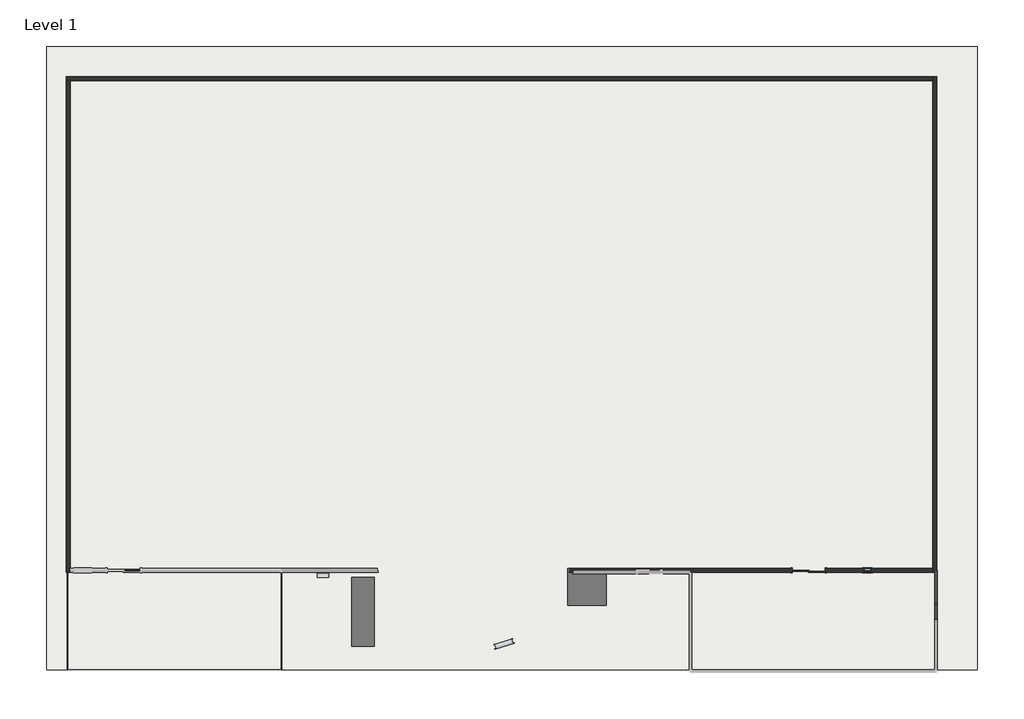
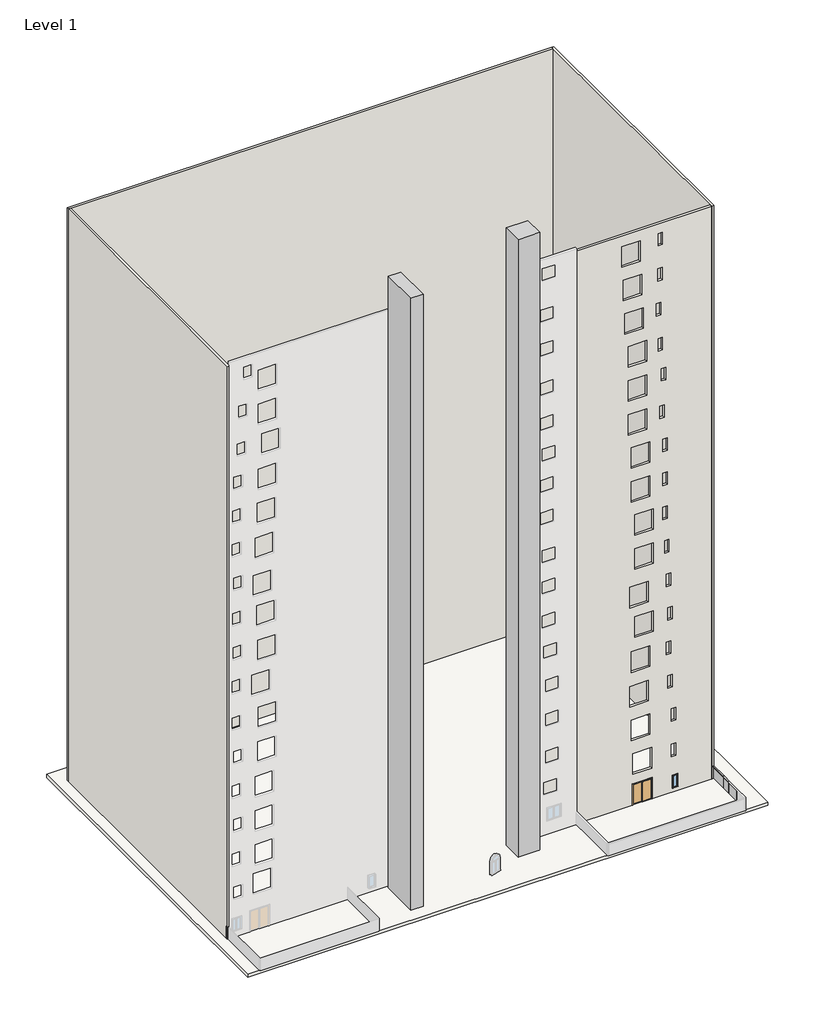
# One storey, part 3 of 3: 4 walls, 3 plates, 2 members, 2 proxies, 1 door, 1 slab, 1 window.
"""IFC4 building model written with IfcOpenShell, lengths in millimetres."""

from ifc_helpers import new_model, si_unit, frame, origin, place, context, project, spatial, polyline, circle_curve, outline, extrude, faceted_brep, transform, mapped, element, save
from ifc_brep_helpers import plane_surface, revolved_surface, advanced_brep
from components import generic_models_1_generic_models_1_ad90d225, generic_models_2_generic_models_2_24f987b9, door_076b30e0, member_ac3a6214, member_afcd4490, system_panel_glazed_8dce6023, system_panel_glazed_2adfbad0, system_panel_glazed_e6c99a0d, window_a765b88f

model = new_model("IFC4")

# Units and contexts
model_context = context("Model", 3, world=origin())
ifc_project = project(units=[si_unit("LENGTHUNIT", "METRE", prefix="MILLI")], contexts=[model_context])

# Site, building, storey
site = spatial("IfcSite", under=ifc_project)
building = spatial("IfcBuilding", under=site)
storey = spatial("IfcBuildingStorey", under=building, Name="Level 1", Elevation=0.0)

# Proxies
placement = place(None, origin())
generic_models_1_generic_models_1_shape = generic_models_1_generic_models_1_ad90d225(model_context)
element("IfcBuildingElementProxy", 1, Name="Generic Models 1 : Generic Models 1", ObjectType="Generic Models 1 : Generic Models 1", at=placement, inside=storey, context=model_context, shape_type="MappedRepresentation", body=[
    mapped(generic_models_1_generic_models_1_shape, transform((0.0, 0.0, 0.0), x_axis=(1.0, 0.0, 0.0), y_axis=(0.0, 1.0, 0.0), z_axis=(0.0, 0.0, 1.0))),
])
generic_models_2_generic_models_2_shape = generic_models_2_generic_models_2_24f987b9(model_context)
element("IfcBuildingElementProxy", 2, Name="Generic Models 2 : Generic Models 2", ObjectType="Generic Models 2 : Generic Models 2", at=placement, inside=storey, context=model_context, shape_type="MappedRepresentation", body=[
    mapped(generic_models_2_generic_models_2_shape, transform((0.0, 0.0, 0.0), x_axis=(1.0, 0.0, 0.0), y_axis=(0.0, 1.0, 0.0), z_axis=(0.0, 0.0, 1.0))),
])

# Door
door_shape = door_076b30e0(model_context)
element("IfcDoor", 3, ObjectType="Door-Double-Sliding : 68\" x 80\"", at=placement, inside=storey, context=model_context, shape_type="MappedRepresentation", body=[
    mapped(door_shape, transform((18835.014721, -12227.7237084, 0.0), x_axis=(-1.0, 0.0, 0.0), y_axis=(0.0, -1.0, 0.0), z_axis=(0.0, 0.0, 1.0))),
])

# Members
member_shape = member_ac3a6214(model_context)
element("IfcMember", 4, ObjectType="Rectangular Mullion : 2.5\" x 5\" rectangular", at=placement, inside=storey, context=model_context, shape_type="MappedRepresentation", body=[
    mapped(member_shape, transform((25464.414721, -14075.656218, 1219.2), x_axis=(0.0, 0.0, 1.0), y_axis=(-1.0, 0.0, 0.0), z_axis=(0.0, -1.0, 0.0))),
])
member_2_shape = member_afcd4490(model_context)
element("IfcMember", 5, ObjectType="Rectangular Mullion : 2.5\" x 5\" rectangular", at=placement, inside=storey, context=model_context, shape_type="MappedRepresentation", body=[
    mapped(member_2_shape, transform((25464.414721, -14936.1224728, 1219.2), x_axis=(0.0, 0.0, 1.0), y_axis=(-1.0, 0.0, 0.0), z_axis=(0.0, -1.0, 0.0))),
])

# Plates
system_panel_glazed_shape = system_panel_glazed_8dce6023(model_context)
element("IfcPlate", 6, ObjectType="System Panel : Glazed", at=placement, inside=storey, context=model_context, shape_type="MappedRepresentation", body=[
    mapped(system_panel_glazed_shape, transform((25464.414721, -13215.1899632, 0.0), x_axis=(0.0, -1.0, 0.0), y_axis=(1.0, 0.0, 0.0), z_axis=(0.0, 0.0, 1.0))),
])
system_panel_glazed_2_shape = system_panel_glazed_2adfbad0(model_context)
element("IfcPlate", 7, ObjectType="System Panel : Glazed", at=placement, inside=storey, context=model_context, shape_type="MappedRepresentation", body=[
    mapped(system_panel_glazed_2_shape, transform((25464.414721, -15581.4721639, 0.0), x_axis=(0.0, -1.0, 0.0), y_axis=(1.0, 0.0, 0.0), z_axis=(0.0, 0.0, 1.0))),
])
system_panel_glazed_3_shape = system_panel_glazed_e6c99a0d(model_context)
element("IfcPlate", 8, ObjectType="System Panel : Glazed", at=placement, inside=storey, context=model_context, shape_type="MappedRepresentation", body=[
    mapped(system_panel_glazed_3_shape, transform((25464.414721, -14505.8893454, 0.0), x_axis=(0.0, -1.0, 0.0), y_axis=(1.0, 0.0, 0.0), z_axis=(0.0, 0.0, 1.0))),
])

# Slab
element("IfcSlab", 9, ObjectType="Generic - 12\"", at=placement, inside=storey, context=model_context, shape_type="SweptSolid", body=[
    extrude(outline(polyline([(27613.7744519, 14926.278145), (27613.7744519, -17534.921855), (-20849.4255481, -17534.921855), (-20849.4255481, 14926.278145), (27613.7744519, 14926.278145)])), frame((0.0, 0.0, -304.8), z_axis=(0.0, 0.0, 1.0), x_axis=(1.0, 0.0, 0.0)), (0.0, 0.0, 1.0), 304.8),
])

# Walls
element("IfcWall", 10, ObjectType="Generic - 8\"", at=placement, inside=storey, context=model_context, shape_type="Brep", body=[
    faceted_brep([(-19823.785279, 13146.8762916, 0.0), (-19620.585279, 13146.8762916, 0.0), (25286.614721, 13146.8762916, 0.0), (25286.614721, 13146.8762916, 56425.3367162), (-19620.585279, 13146.8762916, 56425.3367162), (-19823.785279, 13146.8762916, 56425.3367162), (-19823.785279, 13350.0762916, 0.0), (-19823.785279, 13350.0762916, 56425.3367162), (25286.614721, 13350.0762916, 56425.3367162), (25286.614721, 13350.0762916, 0.0)], [[[0, 1, 2, 3, 4, 5]], [[6, 7, 8, 9]], [[2, 1, 0, 6, 9]], [[5, 4, 3, 8, 7]], [[0, 5, 7, 6]], [[3, 2, 9, 8]]]),
])
element("IfcWall", 11, ObjectType="Generic - 8\"", at=placement, inside=storey, context=model_context, shape_type="Brep", body=[
    faceted_brep([(-19620.585279, -12456.3237084, 0.0), (-19620.585279, -12253.1237084, 0.0), (-19620.585279, 13146.8762916, 0.0), (-19620.585279, 13146.8762916, 56425.3367162), (-19620.585279, -12456.3237084, 56425.3367162), (-19823.785279, -12456.3237084, 0.0), (-19823.785279, -12456.3237084, 56425.3367162), (-19823.785279, 13146.8762916, 56425.3367162), (-19823.785279, 13146.8762916, 0.0)], [[[0, 1, 2, 3, 4]], [[5, 6, 7, 8]], [[2, 1, 0, 5, 8]], [[4, 3, 7, 6]], [[0, 4, 6, 5]], [[3, 2, 8, 7]]]),
])
element("IfcWall", 12, ObjectType="Generic - 8\"", at=placement, inside=storey, context=model_context, shape_type="Brep", body=[
    faceted_brep([(25286.614721, 13350.0762916, 0.0), (25286.614721, 13146.8762916, 0.0), (25286.614721, -12253.1237084, 0.0), (25286.614721, -12456.3237084, 0.0), (25286.614721, -12456.3237084, 56425.3367162), (25286.614721, -12253.1237084, 56425.3367162), (25286.614721, 13146.8762916, 56425.3367162), (25286.614721, 13350.0762916, 56425.3367162), (25489.814721, 13350.0762916, 0.0), (25489.814721, 13350.0762916, 56425.3367162), (25489.814721, -12456.3237084, 56425.3367162), (25489.814721, -12456.3237084, 0.0)], [[[0, 1, 2, 3, 4, 5, 6, 7]], [[8, 9, 10, 11]], [[3, 2, 1, 0, 8, 11]], [[7, 6, 5, 4, 10, 9]], [[0, 7, 9, 8]], [[4, 3, 11, 10]]]),
])
element("IfcWall", 13, ObjectType="Generic - 8\"", at=placement, inside=storey, context=model_context, shape_type="AdvancedBrep", body=[
    advanced_brep(
    [(17971.414721, -12253.1237084, 2032.0), (17971.414721, -12253.1237084, 0.0), (6408.3657946, -12253.1237084, 0.0), (6408.3657946, -12253.1237084, 56425.3367162), (25286.614721, -12253.1237084, 56425.3367162), (25286.614721, -12253.1237084, 0.0), (19698.614721, -12253.1237084, 0.0), (19698.614721, -12253.1237084, 2032.0), (18631.814721, -12253.1237084, 55372.0), (16904.614721, -12253.1237084, 55372.0), (16904.614721, -12253.1237084, 53340.0), (18631.814721, -12253.1237084, 53340.0), (18784.214721, -12253.1237084, 52019.2), (17057.014721, -12253.1237084, 52019.2), (17057.014721, -12253.1237084, 49987.2), (18784.214721, -12253.1237084, 49987.2), (18936.614721, -12253.1237084, 48666.4), (17209.414721, -12253.1237084, 48666.4), (17209.414721, -12253.1237084, 46634.4), (18936.614721, -12253.1237084, 46634.4), (19241.414721, -12253.1237084, 45313.6), (17514.214721, -12253.1237084, 45313.6), (17514.214721, -12253.1237084, 43281.6), (19241.414721, -12253.1237084, 43281.6), (19241.414721, -12253.1237084, 41960.8), (17514.214721, -12253.1237084, 41960.8), (17514.214721, -12253.1237084, 39928.8), (19241.414721, -12253.1237084, 39928.8), (19241.414721, -12253.1237084, 38608.0), (17514.214721, -12253.1237084, 38608.0), (17514.214721, -12253.1237084, 36576.0), (19241.414721, -12253.1237084, 36576.0), (19546.214721, -12253.1237084, 35255.2), (17819.014721, -12253.1237084, 35255.2), (17819.014721, -12253.1237084, 33223.2), (19546.214721, -12253.1237084, 33223.2), (19546.214721, -12253.1237084, 31902.4), (17819.014721, -12253.1237084, 31902.4), (17819.014721, -12253.1237084, 29870.4), (19546.214721, -12253.1237084, 29870.4), (19851.014721, -12253.1237084, 25196.8), (18123.814721, -12253.1237084, 25196.8), (18123.814721, -12253.1237084, 23164.8), (19851.014721, -12253.1237084, 23164.8), (19393.814721, -12253.1237084, 21539.2), (17666.614721, -12253.1237084, 21539.2), (17666.614721, -12253.1237084, 19507.2), (19393.814721, -12253.1237084, 19507.2), (19851.014721, -12253.1237084, 28549.6), (18123.814721, -12253.1237084, 28549.6), (18123.814721, -12253.1237084, 26517.6), (19851.014721, -12253.1237084, 26517.6), (19851.014721, -12253.1237084, 18491.2), (18123.814721, -12253.1237084, 18491.2), (18123.814721, -12253.1237084, 16459.2), (19851.014721, -12253.1237084, 16459.2), (19546.214721, -12253.1237084, 15138.4), (17819.014721, -12253.1237084, 15138.4), (17819.014721, -12253.1237084, 13106.4), (19546.214721, -12253.1237084, 13106.4), (19393.814721, -12253.1237084, 11785.6), (17666.614721, -12253.1237084, 11785.6), (17666.614721, -12253.1237084, 9753.6), (19393.814721, -12253.1237084, 9753.6), (19546.214721, -12253.1237084, 8432.8), (17819.014721, -12253.1237084, 8432.8), (17819.014721, -12253.1237084, 6400.8), (19546.214721, -12253.1237084, 6400.8), (19698.614721, -12253.1237084, 5080.0), (17971.414721, -12253.1237084, 5080.0), (17971.414721, -12253.1237084, 3048.0), (19698.614721, -12253.1237084, 3048.0), (20308.214721, -12253.1237084, 55473.6), (20308.214721, -12253.1237084, 54254.4), (20714.614721, -12253.1237084, 54254.4), (20714.614721, -12253.1237084, 55473.6), (20282.814721, -12253.1237084, 52022.3677442), (20282.814721, -12253.1237084, 50803.1677442), (20689.214721, -12253.1237084, 50803.1677442), (20689.214721, -12253.1237084, 52022.3677442), (20155.814721, -12253.1237084, 48604.1519596), (20155.814721, -12253.1237084, 47384.9519596), (20562.214721, -12253.1237084, 47384.9519596), (20562.214721, -12253.1237084, 48604.1519596), (20308.214721, -12253.1237084, 45110.4), (20308.214721, -12253.1237084, 43891.2), (20714.614721, -12253.1237084, 43891.2), (20714.614721, -12253.1237084, 45110.4), (20613.014721, -12253.1237084, 42062.4), (20613.014721, -12253.1237084, 40843.2), (21019.414721, -12253.1237084, 40843.2), (21019.414721, -12253.1237084, 42062.4), (20460.614721, -12253.1237084, 38404.8), (20460.614721, -12253.1237084, 37185.6), (20867.014721, -12253.1237084, 37185.6), (20867.014721, -12253.1237084, 38404.8), (20765.414721, -12253.1237084, 35052.0), (20765.414721, -12253.1237084, 33832.8), (21171.814721, -12253.1237084, 33832.8), (21171.814721, -12253.1237084, 35052.0), (20765.414721, -12253.1237084, 31699.2), (20765.414721, -12253.1237084, 30480.0), (21171.814721, -12253.1237084, 30480.0), (21171.814721, -12253.1237084, 31699.2), (20765.414721, -12253.1237084, 28346.4), (20765.414721, -12253.1237084, 27127.2), (21171.814721, -12253.1237084, 27127.2), (21171.814721, -12253.1237084, 28346.4), (20917.814721, -12253.1237084, 24993.6), (20917.814721, -12253.1237084, 23774.4), (21324.214721, -12253.1237084, 23774.4), (21324.214721, -12253.1237084, 24993.6), (21070.214721, -12253.1237084, 21640.8), (21070.214721, -12253.1237084, 20421.6), (21476.614721, -12253.1237084, 20421.6), (21476.614721, -12253.1237084, 21640.8), (21222.614721, -12253.1237084, 18288.0), (21222.614721, -12253.1237084, 17068.8), (21629.014721, -12253.1237084, 17068.8), (21629.014721, -12253.1237084, 18288.0), (21070.214721, -12253.1237084, 14935.2), (21070.214721, -12253.1237084, 13716.0), (21476.614721, -12253.1237084, 13716.0), (21476.614721, -12253.1237084, 14935.2), (21222.614721, -12253.1237084, 11582.4), (21222.614721, -12253.1237084, 10363.2), (21629.014721, -12253.1237084, 10363.2), (21629.014721, -12253.1237084, 11582.4), (21527.414721, -12253.1237084, 8229.6), (21527.414721, -12253.1237084, 7010.4), (21933.814721, -12253.1237084, 7010.4), (21933.814721, -12253.1237084, 8229.6), (21527.414721, -12253.1237084, 4734.0057153), (21527.414721, -12253.1237084, 3514.8057153), (21933.814721, -12253.1237084, 3514.8057153), (21933.814721, -12253.1237084, 4734.0057153), (21679.814721, -12253.1237084, 1610.6543351), (21679.814721, -12253.1237084, 391.4543351), (22086.214721, -12253.1237084, 391.4543351), (22086.214721, -12253.1237084, 1610.6543351), (6362.4838197, -12456.3237084, 0.0), (6571.5594464, -12456.3237084, 0.0), (17971.414721, -12456.3237084, 0.0), (17971.414721, -12456.3237084, 2032.0), (19698.614721, -12456.3237084, 2032.0), (19698.614721, -12456.3237084, 0.0), (25286.614721, -12456.3237084, 0.0), (25286.614721, -12456.3237084, 56425.3367162), (6571.5594464, -12456.3237084, 56425.3367162), (6362.4838197, -12456.3237084, 56425.3367162), (18631.814721, -12456.3237084, 55372.0), (18631.814721, -12456.3237084, 53340.0), (16904.614721, -12456.3237084, 53340.0), (16904.614721, -12456.3237084, 55372.0), (18784.214721, -12456.3237084, 52019.2), (18784.214721, -12456.3237084, 49987.2), (17057.014721, -12456.3237084, 49987.2), (17057.014721, -12456.3237084, 52019.2), (18936.614721, -12456.3237084, 48666.4), (18936.614721, -12456.3237084, 46634.4), (17209.414721, -12456.3237084, 46634.4), (17209.414721, -12456.3237084, 48666.4), (19241.414721, -12456.3237084, 45313.6), (19241.414721, -12456.3237084, 43281.6), (17514.214721, -12456.3237084, 43281.6), (17514.214721, -12456.3237084, 45313.6), (19241.414721, -12456.3237084, 41960.8), (19241.414721, -12456.3237084, 39928.8), (17514.214721, -12456.3237084, 39928.8), (17514.214721, -12456.3237084, 41960.8), (19241.414721, -12456.3237084, 38608.0), (19241.414721, -12456.3237084, 36576.0), (17514.214721, -12456.3237084, 36576.0), (17514.214721, -12456.3237084, 38608.0), (19546.214721, -12456.3237084, 35255.2), (19546.214721, -12456.3237084, 33223.2), (17819.014721, -12456.3237084, 33223.2), (17819.014721, -12456.3237084, 35255.2), (19546.214721, -12456.3237084, 31902.4), (19546.214721, -12456.3237084, 29870.4), (17819.014721, -12456.3237084, 29870.4), (17819.014721, -12456.3237084, 31902.4), (19851.014721, -12456.3237084, 25196.8), (19851.014721, -12456.3237084, 23164.8), (18123.814721, -12456.3237084, 23164.8), (18123.814721, -12456.3237084, 25196.8), (19393.814721, -12456.3237084, 21539.2), (19393.814721, -12456.3237084, 19507.2), (17666.614721, -12456.3237084, 19507.2), (17666.614721, -12456.3237084, 21539.2), (19851.014721, -12456.3237084, 28549.6), (19851.014721, -12456.3237084, 26517.6), (18123.814721, -12456.3237084, 26517.6), (18123.814721, -12456.3237084, 28549.6), (19851.014721, -12456.3237084, 18491.2), (19851.014721, -12456.3237084, 16459.2), (18123.814721, -12456.3237084, 16459.2), (18123.814721, -12456.3237084, 18491.2), (19546.214721, -12456.3237084, 15138.4), (19546.214721, -12456.3237084, 13106.4), (17819.014721, -12456.3237084, 13106.4), (17819.014721, -12456.3237084, 15138.4), (19393.814721, -12456.3237084, 11785.6), (19393.814721, -12456.3237084, 9753.6), (17666.614721, -12456.3237084, 9753.6), (17666.614721, -12456.3237084, 11785.6), (19546.214721, -12456.3237084, 8432.8), (19546.214721, -12456.3237084, 6400.8), (17819.014721, -12456.3237084, 6400.8), (17819.014721, -12456.3237084, 8432.8), (19698.614721, -12456.3237084, 5080.0), (19698.614721, -12456.3237084, 3048.0), (17971.414721, -12456.3237084, 3048.0), (17971.414721, -12456.3237084, 5080.0), (20308.214721, -12456.3237084, 55473.6), (20714.614721, -12456.3237084, 55473.6), (20714.614721, -12456.3237084, 54254.4), (20308.214721, -12456.3237084, 54254.4), (20282.814721, -12456.3237084, 52022.3677442), (20689.214721, -12456.3237084, 52022.3677442), (20689.214721, -12456.3237084, 50803.1677442), (20282.814721, -12456.3237084, 50803.1677442), (20155.814721, -12456.3237084, 48604.1519596), (20562.214721, -12456.3237084, 48604.1519596), (20562.214721, -12456.3237084, 47384.9519596), (20155.814721, -12456.3237084, 47384.9519596), (20308.214721, -12456.3237084, 45110.4), (20714.614721, -12456.3237084, 45110.4), (20714.614721, -12456.3237084, 43891.2), (20308.214721, -12456.3237084, 43891.2), (20613.014721, -12456.3237084, 42062.4), (21019.414721, -12456.3237084, 42062.4), (21019.414721, -12456.3237084, 40843.2), (20613.014721, -12456.3237084, 40843.2), (20460.614721, -12456.3237084, 38404.8), (20867.014721, -12456.3237084, 38404.8), (20867.014721, -12456.3237084, 37185.6), (20460.614721, -12456.3237084, 37185.6), (20765.414721, -12456.3237084, 35052.0), (21171.814721, -12456.3237084, 35052.0), (21171.814721, -12456.3237084, 33832.8), (20765.414721, -12456.3237084, 33832.8), (20765.414721, -12456.3237084, 31699.2), (21171.814721, -12456.3237084, 31699.2), (21171.814721, -12456.3237084, 30480.0), (20765.414721, -12456.3237084, 30480.0), (20765.414721, -12456.3237084, 28346.4), (21171.814721, -12456.3237084, 28346.4), (21171.814721, -12456.3237084, 27127.2), (20765.414721, -12456.3237084, 27127.2), (20917.814721, -12456.3237084, 24993.6), (21324.214721, -12456.3237084, 24993.6), (21324.214721, -12456.3237084, 23774.4), (20917.814721, -12456.3237084, 23774.4), (21070.214721, -12456.3237084, 21640.8), (21476.614721, -12456.3237084, 21640.8), (21476.614721, -12456.3237084, 20421.6), (21070.214721, -12456.3237084, 20421.6), (21222.614721, -12456.3237084, 18288.0), (21629.014721, -12456.3237084, 18288.0), (21629.014721, -12456.3237084, 17068.8), (21222.614721, -12456.3237084, 17068.8), (21070.214721, -12456.3237084, 14935.2), (21476.614721, -12456.3237084, 14935.2), (21476.614721, -12456.3237084, 13716.0), (21070.214721, -12456.3237084, 13716.0), (21222.614721, -12456.3237084, 11582.4), (21629.014721, -12456.3237084, 11582.4), (21629.014721, -12456.3237084, 10363.2), (21222.614721, -12456.3237084, 10363.2), (21527.414721, -12456.3237084, 8229.6), (21933.814721, -12456.3237084, 8229.6), (21933.814721, -12456.3237084, 7010.4), (21527.414721, -12456.3237084, 7010.4), (21527.414721, -12456.3237084, 4734.0057153), (21933.814721, -12456.3237084, 4734.0057153), (21933.814721, -12456.3237084, 3514.8057153), (21527.414721, -12456.3237084, 3514.8057153), (21679.814721, -12456.3237084, 1610.6543351), (22086.214721, -12456.3237084, 1610.6543351), (22086.214721, -12456.3237084, 391.4543351), (21679.814721, -12456.3237084, 391.4543351), (6386.5095252, -12354.7237244, 56425.3367162)],
    [
        (0, 1),
        (1, 2),
        (2, 3),
        (3, 4),
        (4, 5),
        (5, 6),
        (6, 7),
        (7, 0),
        (8, 9),
        (9, 10),
        (10, 11),
        (11, 8),
        (12, 13),
        (13, 14),
        (14, 15),
        (15, 12),
        (16, 17),
        (17, 18),
        (18, 19),
        (19, 16),
        (20, 21),
        (21, 22),
        (22, 23),
        (23, 20),
        (24, 25),
        (25, 26),
        (26, 27),
        (27, 24),
        (28, 29),
        (29, 30),
        (30, 31),
        (31, 28),
        (32, 33),
        (33, 34),
        (34, 35),
        (35, 32),
        (36, 37),
        (37, 38),
        (38, 39),
        (39, 36),
        (40, 41),
        (41, 42),
        (42, 43),
        (43, 40),
        (44, 45),
        (45, 46),
        (46, 47),
        (47, 44),
        (48, 49),
        (49, 50),
        (50, 51),
        (51, 48),
        (52, 53),
        (53, 54),
        (54, 55),
        (55, 52),
        (56, 57),
        (57, 58),
        (58, 59),
        (59, 56),
        (60, 61),
        (61, 62),
        (62, 63),
        (63, 60),
        (64, 65),
        (65, 66),
        (66, 67),
        (67, 64),
        (68, 69),
        (69, 70),
        (70, 71),
        (71, 68),
        (72, 73),
        (73, 74),
        (74, 75),
        (75, 72),
        (76, 77),
        (77, 78),
        (78, 79),
        (79, 76),
        (80, 81),
        (81, 82),
        (82, 83),
        (83, 80),
        (84, 85),
        (85, 86),
        (86, 87),
        (87, 84),
        (88, 89),
        (89, 90),
        (90, 91),
        (91, 88),
        (92, 93),
        (93, 94),
        (94, 95),
        (95, 92),
        (96, 97),
        (97, 98),
        (98, 99),
        (99, 96),
        (100, 101),
        (101, 102),
        (102, 103),
        (103, 100),
        (104, 105),
        (105, 106),
        (106, 107),
        (107, 104),
        (108, 109),
        (109, 110),
        (110, 111),
        (111, 108),
        (112, 113),
        (113, 114),
        (114, 115),
        (115, 112),
        (116, 117),
        (117, 118),
        (118, 119),
        (119, 116),
        (120, 121),
        (121, 122),
        (122, 123),
        (123, 120),
        (124, 125),
        (125, 126),
        (126, 127),
        (127, 124),
        (128, 129),
        (129, 130),
        (130, 131),
        (131, 128),
        (132, 133),
        (133, 134),
        (134, 135),
        (135, 132),
        (136, 137),
        (137, 138),
        (138, 139),
        (139, 136),
        (140, 141),
        (141, 142),
        (142, 143),
        (143, 144),
        (144, 145),
        (145, 146),
        (146, 147),
        (147, 148),
        (148, 149),
        (149, 140),
        (150, 151),
        (151, 152),
        (152, 153),
        (153, 150),
        (154, 155),
        (155, 156),
        (156, 157),
        (157, 154),
        (158, 159),
        (159, 160),
        (160, 161),
        (161, 158),
        (162, 163),
        (163, 164),
        (164, 165),
        (165, 162),
        (166, 167),
        (167, 168),
        (168, 169),
        (169, 166),
        (170, 171),
        (171, 172),
        (172, 173),
        (173, 170),
        (174, 175),
        (175, 176),
        (176, 177),
        (177, 174),
        (178, 179),
        (179, 180),
        (180, 181),
        (181, 178),
        (182, 183),
        (183, 184),
        (184, 185),
        (185, 182),
        (186, 187),
        (187, 188),
        (188, 189),
        (189, 186),
        (190, 191),
        (191, 192),
        (192, 193),
        (193, 190),
        (194, 195),
        (195, 196),
        (196, 197),
        (197, 194),
        (198, 199),
        (199, 200),
        (200, 201),
        (201, 198),
        (202, 203),
        (203, 204),
        (204, 205),
        (205, 202),
        (206, 207),
        (207, 208),
        (208, 209),
        (209, 206),
        (210, 211),
        (211, 212),
        (212, 213),
        (213, 210),
        (214, 215),
        (215, 216),
        (216, 217),
        (217, 214),
        (218, 219),
        (219, 220),
        (220, 221),
        (221, 218),
        (222, 223),
        (223, 224),
        (224, 225),
        (225, 222),
        (226, 227),
        (227, 228),
        (228, 229),
        (229, 226),
        (230, 231),
        (231, 232),
        (232, 233),
        (233, 230),
        (234, 235),
        (235, 236),
        (236, 237),
        (237, 234),
        (238, 239),
        (239, 240),
        (240, 241),
        (241, 238),
        (242, 243),
        (243, 244),
        (244, 245),
        (245, 242),
        (246, 247),
        (247, 248),
        (248, 249),
        (249, 246),
        (250, 251),
        (251, 252),
        (252, 253),
        (253, 250),
        (254, 255),
        (255, 256),
        (256, 257),
        (257, 254),
        (258, 259),
        (259, 260),
        (260, 261),
        (261, 258),
        (262, 263),
        (263, 264),
        (264, 265),
        (265, 262),
        (266, 267),
        (267, 268),
        (268, 269),
        (269, 266),
        (270, 271),
        (271, 272),
        (272, 273),
        (273, 270),
        (274, 275),
        (275, 276),
        (276, 277),
        (277, 274),
        (278, 279),
        (279, 280),
        (280, 281),
        (281, 278),
        (5, 146),
        (145, 6),
        (1, 142),
        (140, 2, circle_curve(frame((1385.214721, -11225.6906671, 0.0), z_axis=(0.0, 0.0, 1.0), x_axis=(1.0, 0.0, 0.0)), 5127.1498284)),
        (3, 282, circle_curve(frame((1385.214721, -11225.6906671, 56425.3367162), z_axis=(0.0, 0.0, -1.0), x_axis=(1.0, 0.0, 0.0)), 5127.1498284)),
        (282, 149, circle_curve(frame((1385.214721, -11225.6906671, 56425.3367162), z_axis=(0.0, 0.0, -1.0), x_axis=(1.0, 0.0, 0.0)), 5127.1498284)),
        (147, 4),
        (150, 8),
        (11, 151),
        (10, 152),
        (9, 153),
        (154, 12),
        (15, 155),
        (14, 156),
        (13, 157),
        (158, 16),
        (19, 159),
        (18, 160),
        (17, 161),
        (162, 20),
        (23, 163),
        (22, 164),
        (21, 165),
        (166, 24),
        (27, 167),
        (26, 168),
        (25, 169),
        (170, 28),
        (31, 171),
        (30, 172),
        (29, 173),
        (174, 32),
        (35, 175),
        (34, 176),
        (33, 177),
        (178, 36),
        (39, 179),
        (38, 180),
        (37, 181),
        (182, 40),
        (43, 183),
        (42, 184),
        (41, 185),
        (186, 44),
        (47, 187),
        (46, 188),
        (45, 189),
        (190, 48),
        (51, 191),
        (50, 192),
        (49, 193),
        (194, 52),
        (55, 195),
        (54, 196),
        (53, 197),
        (198, 56),
        (59, 199),
        (58, 200),
        (57, 201),
        (202, 60),
        (63, 203),
        (62, 204),
        (61, 205),
        (206, 64),
        (67, 207),
        (66, 208),
        (65, 209),
        (210, 68),
        (71, 211),
        (70, 212),
        (69, 213),
        (144, 7),
        (0, 143),
        (72, 214),
        (217, 73),
        (216, 74),
        (215, 75),
        (76, 218),
        (221, 77),
        (220, 78),
        (219, 79),
        (80, 222),
        (225, 81),
        (224, 82),
        (223, 83),
        (84, 226),
        (229, 85),
        (228, 86),
        (227, 87),
        (88, 230),
        (233, 89),
        (232, 90),
        (231, 91),
        (92, 234),
        (237, 93),
        (236, 94),
        (235, 95),
        (96, 238),
        (241, 97),
        (240, 98),
        (239, 99),
        (100, 242),
        (245, 101),
        (244, 102),
        (243, 103),
        (104, 246),
        (249, 105),
        (248, 106),
        (247, 107),
        (108, 250),
        (253, 109),
        (252, 110),
        (251, 111),
        (112, 254),
        (257, 113),
        (256, 114),
        (255, 115),
        (116, 258),
        (261, 117),
        (260, 118),
        (259, 119),
        (120, 262),
        (265, 121),
        (264, 122),
        (263, 123),
        (124, 266),
        (269, 125),
        (268, 126),
        (267, 127),
        (128, 270),
        (273, 129),
        (272, 130),
        (271, 131),
        (132, 274),
        (277, 133),
        (276, 134),
        (275, 135),
        (136, 278),
        (281, 137),
        (280, 138),
        (279, 139),
    ],
    [
        plane_surface(frame((25388.214721, -12253.1237084, 0.0), z_axis=(0.0, 1.0, 0.0), x_axis=(-1.0, 0.0, 0.0))),
        plane_surface(frame((25388.214721, -12456.3237084, 0.0), z_axis=(0.0, -1.0, 0.0), x_axis=(1.0, 0.0, 0.0))),
        plane_surface(frame((25489.814721, -12253.1237084, 0.0), z_axis=(0.0, 0.0, -1.0), x_axis=(0.0, -1.0, 0.0))),
        plane_surface(frame((6490.614721, -12253.1237084, 56425.3367162), z_axis=(0.0, 0.0, 1.0), x_axis=(0.0, -1.0, 0.0))),
        plane_surface(frame((25286.614721, 13248.4762916, 0.0), z_axis=(1.0, 0.0, 0.0), x_axis=(0.0, -1.0, 0.0))),
        revolved_surface(polyline([(6512.3645494, -11225.6906671, 0.0), (6512.3645494, -11225.6906671, 56425.3367162)]), (1385.214721, -11225.6906671, 0.0), (0.0, 0.0, -1.0)),
        plane_surface(frame((18631.814721, -12456.3237084, 55372.0), z_axis=(-1.0, 0.0, 0.0), x_axis=(0.0, 1.0, 0.0))),
        plane_surface(frame((18631.814721, -12456.3237084, 53340.0), z_axis=(0.0, 0.0, 1.0), x_axis=(0.0, 1.0, 0.0))),
        plane_surface(frame((16904.614721, -12456.3237084, 53340.0), z_axis=(1.0, 0.0, 0.0), x_axis=(0.0, 1.0, 0.0))),
        plane_surface(frame((16904.614721, -12456.3237084, 55372.0), z_axis=(0.0, 0.0, -1.0), x_axis=(0.0, 1.0, 0.0))),
        plane_surface(frame((18784.214721, -12456.3237084, 52019.2), z_axis=(-1.0, 0.0, 0.0), x_axis=(0.0, 1.0, 0.0))),
        plane_surface(frame((18784.214721, -12456.3237084, 49987.2), z_axis=(0.0, 0.0, 1.0), x_axis=(0.0, 1.0, 0.0))),
        plane_surface(frame((17057.014721, -12456.3237084, 49987.2), z_axis=(1.0, 0.0, 0.0), x_axis=(0.0, 1.0, 0.0))),
        plane_surface(frame((17057.014721, -12456.3237084, 52019.2), z_axis=(0.0, 0.0, -1.0), x_axis=(0.0, 1.0, 0.0))),
        plane_surface(frame((18936.614721, -12456.3237084, 48666.4), z_axis=(-1.0, 0.0, 0.0), x_axis=(0.0, 1.0, 0.0))),
        plane_surface(frame((18936.614721, -12456.3237084, 46634.4), z_axis=(0.0, 0.0, 1.0), x_axis=(0.0, 1.0, 0.0))),
        plane_surface(frame((17209.414721, -12456.3237084, 46634.4), z_axis=(1.0, 0.0, 0.0), x_axis=(0.0, 1.0, 0.0))),
        plane_surface(frame((17209.414721, -12456.3237084, 48666.4), z_axis=(0.0, 0.0, -1.0), x_axis=(0.0, 1.0, 0.0))),
        plane_surface(frame((19241.414721, -12456.3237084, 45313.6), z_axis=(-1.0, 0.0, 0.0), x_axis=(0.0, 1.0, 0.0))),
        plane_surface(frame((19241.414721, -12456.3237084, 43281.6), z_axis=(0.0, 0.0, 1.0), x_axis=(0.0, 1.0, 0.0))),
        plane_surface(frame((17514.214721, -12456.3237084, 43281.6), z_axis=(1.0, 0.0, 0.0), x_axis=(0.0, 1.0, 0.0))),
        plane_surface(frame((17514.214721, -12456.3237084, 45313.6), z_axis=(0.0, 0.0, -1.0), x_axis=(0.0, 1.0, 0.0))),
        plane_surface(frame((19241.414721, -12456.3237084, 41960.8), z_axis=(-1.0, 0.0, 0.0), x_axis=(0.0, 1.0, 0.0))),
        plane_surface(frame((19241.414721, -12456.3237084, 39928.8), z_axis=(0.0, 0.0, 1.0), x_axis=(0.0, 1.0, 0.0))),
        plane_surface(frame((17514.214721, -12456.3237084, 39928.8), z_axis=(1.0, 0.0, 0.0), x_axis=(0.0, 1.0, 0.0))),
        plane_surface(frame((17514.214721, -12456.3237084, 41960.8), z_axis=(0.0, 0.0, -1.0), x_axis=(0.0, 1.0, 0.0))),
        plane_surface(frame((19241.414721, -12456.3237084, 38608.0), z_axis=(-1.0, 0.0, 0.0), x_axis=(0.0, 1.0, 0.0))),
        plane_surface(frame((19241.414721, -12456.3237084, 36576.0), z_axis=(0.0, 0.0, 1.0), x_axis=(0.0, 1.0, 0.0))),
        plane_surface(frame((17514.214721, -12456.3237084, 36576.0), z_axis=(1.0, 0.0, 0.0), x_axis=(0.0, 1.0, 0.0))),
        plane_surface(frame((17514.214721, -12456.3237084, 38608.0), z_axis=(0.0, 0.0, -1.0), x_axis=(0.0, 1.0, 0.0))),
        plane_surface(frame((19546.214721, -12456.3237084, 35255.2), z_axis=(-1.0, 0.0, 0.0), x_axis=(0.0, 1.0, 0.0))),
        plane_surface(frame((19546.214721, -12456.3237084, 33223.2), z_axis=(0.0, 0.0, 1.0), x_axis=(0.0, 1.0, 0.0))),
        plane_surface(frame((17819.014721, -12456.3237084, 33223.2), z_axis=(1.0, 0.0, 0.0), x_axis=(0.0, 1.0, 0.0))),
        plane_surface(frame((17819.014721, -12456.3237084, 35255.2), z_axis=(0.0, 0.0, -1.0), x_axis=(0.0, 1.0, 0.0))),
        plane_surface(frame((19546.214721, -12456.3237084, 31902.4), z_axis=(-1.0, 0.0, 0.0), x_axis=(0.0, 1.0, 0.0))),
        plane_surface(frame((19546.214721, -12456.3237084, 29870.4), z_axis=(0.0, 0.0, 1.0), x_axis=(0.0, 1.0, 0.0))),
        plane_surface(frame((17819.014721, -12456.3237084, 29870.4), z_axis=(1.0, 0.0, 0.0), x_axis=(0.0, 1.0, 0.0))),
        plane_surface(frame((17819.014721, -12456.3237084, 31902.4), z_axis=(0.0, 0.0, -1.0), x_axis=(0.0, 1.0, 0.0))),
        plane_surface(frame((19851.014721, -12456.3237084, 25196.8), z_axis=(-1.0, 0.0, 0.0), x_axis=(0.0, 1.0, 0.0))),
        plane_surface(frame((19851.014721, -12456.3237084, 23164.8), z_axis=(0.0, 0.0, 1.0), x_axis=(0.0, 1.0, 0.0))),
        plane_surface(frame((18123.814721, -12456.3237084, 23164.8), z_axis=(1.0, 0.0, 0.0), x_axis=(0.0, 1.0, 0.0))),
        plane_surface(frame((18123.814721, -12456.3237084, 25196.8), z_axis=(0.0, 0.0, -1.0), x_axis=(0.0, 1.0, 0.0))),
        plane_surface(frame((19393.814721, -12456.3237084, 21539.2), z_axis=(-1.0, 0.0, 0.0), x_axis=(0.0, 1.0, 0.0))),
        plane_surface(frame((19393.814721, -12456.3237084, 19507.2), z_axis=(0.0, 0.0, 1.0), x_axis=(0.0, 1.0, 0.0))),
        plane_surface(frame((17666.614721, -12456.3237084, 19507.2), z_axis=(1.0, 0.0, 0.0), x_axis=(0.0, 1.0, 0.0))),
        plane_surface(frame((17666.614721, -12456.3237084, 21539.2), z_axis=(0.0, 0.0, -1.0), x_axis=(0.0, 1.0, 0.0))),
        plane_surface(frame((19851.014721, -12456.3237084, 28549.6), z_axis=(-1.0, 0.0, 0.0), x_axis=(0.0, 1.0, 0.0))),
        plane_surface(frame((19851.014721, -12456.3237084, 26517.6), z_axis=(0.0, 0.0, 1.0), x_axis=(0.0, 1.0, 0.0))),
        plane_surface(frame((18123.814721, -12456.3237084, 26517.6), z_axis=(1.0, 0.0, 0.0), x_axis=(0.0, 1.0, 0.0))),
        plane_surface(frame((18123.814721, -12456.3237084, 28549.6), z_axis=(0.0, 0.0, -1.0), x_axis=(0.0, 1.0, 0.0))),
        plane_surface(frame((19851.014721, -12456.3237084, 18491.2), z_axis=(-1.0, 0.0, 0.0), x_axis=(0.0, 1.0, 0.0))),
        plane_surface(frame((19851.014721, -12456.3237084, 16459.2), z_axis=(0.0, 0.0, 1.0), x_axis=(0.0, 1.0, 0.0))),
        plane_surface(frame((18123.814721, -12456.3237084, 16459.2), z_axis=(1.0, 0.0, 0.0), x_axis=(0.0, 1.0, 0.0))),
        plane_surface(frame((18123.814721, -12456.3237084, 18491.2), z_axis=(0.0, 0.0, -1.0), x_axis=(0.0, 1.0, 0.0))),
        plane_surface(frame((19546.214721, -12456.3237084, 15138.4), z_axis=(-1.0, 0.0, 0.0), x_axis=(0.0, 1.0, 0.0))),
        plane_surface(frame((19546.214721, -12456.3237084, 13106.4), z_axis=(0.0, 0.0, 1.0), x_axis=(0.0, 1.0, 0.0))),
        plane_surface(frame((17819.014721, -12456.3237084, 13106.4), z_axis=(1.0, 0.0, 0.0), x_axis=(0.0, 1.0, 0.0))),
        plane_surface(frame((17819.014721, -12456.3237084, 15138.4), z_axis=(0.0, 0.0, -1.0), x_axis=(0.0, 1.0, 0.0))),
        plane_surface(frame((19393.814721, -12456.3237084, 11785.6), z_axis=(-1.0, 0.0, 0.0), x_axis=(0.0, 1.0, 0.0))),
        plane_surface(frame((19393.814721, -12456.3237084, 9753.6), z_axis=(0.0, 0.0, 1.0), x_axis=(0.0, 1.0, 0.0))),
        plane_surface(frame((17666.614721, -12456.3237084, 9753.6), z_axis=(1.0, 0.0, 0.0), x_axis=(0.0, 1.0, 0.0))),
        plane_surface(frame((17666.614721, -12456.3237084, 11785.6), z_axis=(0.0, 0.0, -1.0), x_axis=(0.0, 1.0, 0.0))),
        plane_surface(frame((19546.214721, -12456.3237084, 8432.8), z_axis=(-1.0, 0.0, 0.0), x_axis=(0.0, 1.0, 0.0))),
        plane_surface(frame((19546.214721, -12456.3237084, 6400.8), z_axis=(0.0, 0.0, 1.0), x_axis=(0.0, 1.0, 0.0))),
        plane_surface(frame((17819.014721, -12456.3237084, 6400.8), z_axis=(1.0, 0.0, 0.0), x_axis=(0.0, 1.0, 0.0))),
        plane_surface(frame((17819.014721, -12456.3237084, 8432.8), z_axis=(0.0, 0.0, -1.0), x_axis=(0.0, 1.0, 0.0))),
        plane_surface(frame((19698.614721, -12456.3237084, 5080.0), z_axis=(-1.0, 0.0, 0.0), x_axis=(0.0, 1.0, 0.0))),
        plane_surface(frame((19698.614721, -12456.3237084, 3048.0), z_axis=(0.0, 0.0, 1.0), x_axis=(0.0, 1.0, 0.0))),
        plane_surface(frame((17971.414721, -12456.3237084, 3048.0), z_axis=(1.0, 0.0, 0.0), x_axis=(0.0, 1.0, 0.0))),
        plane_surface(frame((17971.414721, -12456.3237084, 5080.0), z_axis=(0.0, 0.0, -1.0), x_axis=(0.0, 1.0, 0.0))),
        plane_surface(frame((19698.614721, -12456.3237084, 2032.0), z_axis=(-1.0, 0.0, 0.0), x_axis=(0.0, 1.0, 0.0))),
        plane_surface(frame((17971.414721, -12456.3237084, 0.0), z_axis=(1.0, 0.0, 0.0), x_axis=(0.0, 1.0, 0.0))),
        plane_surface(frame((17971.414721, -12456.3237084, 2032.0), z_axis=(0.0, 0.0, -1.0), x_axis=(0.0, 1.0, 0.0))),
        plane_surface(frame((20308.214721, -12253.1237084, 55473.6), z_axis=(1.0, 0.0, 0.0), x_axis=(0.0, -1.0, 0.0))),
        plane_surface(frame((20308.214721, -12253.1237084, 54254.4), z_axis=(0.0, 0.0, 1.0), x_axis=(0.0, -1.0, 0.0))),
        plane_surface(frame((20714.614721, -12253.1237084, 54254.4), z_axis=(-1.0, 0.0, 0.0), x_axis=(0.0, -1.0, 0.0))),
        plane_surface(frame((20714.614721, -12253.1237084, 55473.6), z_axis=(0.0, 0.0, -1.0), x_axis=(0.0, -1.0, 0.0))),
        plane_surface(frame((20282.814721, -12253.1237084, 52022.3677442), z_axis=(1.0, 0.0, 0.0), x_axis=(0.0, -1.0, 0.0))),
        plane_surface(frame((20282.814721, -12253.1237084, 50803.1677442), z_axis=(0.0, 0.0, 1.0), x_axis=(0.0, -1.0, 0.0))),
        plane_surface(frame((20689.214721, -12253.1237084, 50803.1677442), z_axis=(-1.0, 0.0, 0.0), x_axis=(0.0, -1.0, 0.0))),
        plane_surface(frame((20689.214721, -12253.1237084, 52022.3677442), z_axis=(0.0, 0.0, -1.0), x_axis=(0.0, -1.0, 0.0))),
        plane_surface(frame((20155.814721, -12253.1237084, 48604.1519596), z_axis=(1.0, 0.0, 0.0), x_axis=(0.0, -1.0, 0.0))),
        plane_surface(frame((20155.814721, -12253.1237084, 47384.9519596), z_axis=(0.0, 0.0, 1.0), x_axis=(0.0, -1.0, 0.0))),
        plane_surface(frame((20562.214721, -12253.1237084, 47384.9519596), z_axis=(-1.0, 0.0, 0.0), x_axis=(0.0, -1.0, 0.0))),
        plane_surface(frame((20562.214721, -12253.1237084, 48604.1519596), z_axis=(0.0, 0.0, -1.0), x_axis=(0.0, -1.0, 0.0))),
        plane_surface(frame((20308.214721, -12253.1237084, 45110.4), z_axis=(1.0, 0.0, 0.0), x_axis=(0.0, -1.0, 0.0))),
        plane_surface(frame((20308.214721, -12253.1237084, 43891.2), z_axis=(0.0, 0.0, 1.0), x_axis=(0.0, -1.0, 0.0))),
        plane_surface(frame((20714.614721, -12253.1237084, 43891.2), z_axis=(-1.0, 0.0, 0.0), x_axis=(0.0, -1.0, 0.0))),
        plane_surface(frame((20714.614721, -12253.1237084, 45110.4), z_axis=(0.0, 0.0, -1.0), x_axis=(0.0, -1.0, 0.0))),
        plane_surface(frame((20613.014721, -12253.1237084, 42062.4), z_axis=(1.0, 0.0, 0.0), x_axis=(0.0, -1.0, 0.0))),
        plane_surface(frame((20613.014721, -12253.1237084, 40843.2), z_axis=(0.0, 0.0, 1.0), x_axis=(0.0, -1.0, 0.0))),
        plane_surface(frame((21019.414721, -12253.1237084, 40843.2), z_axis=(-1.0, 0.0, 0.0), x_axis=(0.0, -1.0, 0.0))),
        plane_surface(frame((21019.414721, -12253.1237084, 42062.4), z_axis=(0.0, 0.0, -1.0), x_axis=(0.0, -1.0, 0.0))),
        plane_surface(frame((20460.614721, -12253.1237084, 38404.8), z_axis=(1.0, 0.0, 0.0), x_axis=(0.0, -1.0, 0.0))),
        plane_surface(frame((20460.614721, -12253.1237084, 37185.6), z_axis=(0.0, 0.0, 1.0), x_axis=(0.0, -1.0, 0.0))),
        plane_surface(frame((20867.014721, -12253.1237084, 37185.6), z_axis=(-1.0, 0.0, 0.0), x_axis=(0.0, -1.0, 0.0))),
        plane_surface(frame((20867.014721, -12253.1237084, 38404.8), z_axis=(0.0, 0.0, -1.0), x_axis=(0.0, -1.0, 0.0))),
        plane_surface(frame((20765.414721, -12253.1237084, 35052.0), z_axis=(1.0, 0.0, 0.0), x_axis=(0.0, -1.0, 0.0))),
        plane_surface(frame((20765.414721, -12253.1237084, 33832.8), z_axis=(0.0, 0.0, 1.0), x_axis=(0.0, -1.0, 0.0))),
        plane_surface(frame((21171.814721, -12253.1237084, 33832.8), z_axis=(-1.0, 0.0, 0.0), x_axis=(0.0, -1.0, 0.0))),
        plane_surface(frame((21171.814721, -12253.1237084, 35052.0), z_axis=(0.0, 0.0, -1.0), x_axis=(0.0, -1.0, 0.0))),
        plane_surface(frame((20765.414721, -12253.1237084, 31699.2), z_axis=(1.0, 0.0, 0.0), x_axis=(0.0, -1.0, 0.0))),
        plane_surface(frame((20765.414721, -12253.1237084, 30480.0), z_axis=(0.0, 0.0, 1.0), x_axis=(0.0, -1.0, 0.0))),
        plane_surface(frame((21171.814721, -12253.1237084, 30480.0), z_axis=(-1.0, 0.0, 0.0), x_axis=(0.0, -1.0, 0.0))),
        plane_surface(frame((21171.814721, -12253.1237084, 31699.2), z_axis=(0.0, 0.0, -1.0), x_axis=(0.0, -1.0, 0.0))),
        plane_surface(frame((20765.414721, -12253.1237084, 28346.4), z_axis=(1.0, 0.0, 0.0), x_axis=(0.0, -1.0, 0.0))),
        plane_surface(frame((20765.414721, -12253.1237084, 27127.2), z_axis=(0.0, 0.0, 1.0), x_axis=(0.0, -1.0, 0.0))),
        plane_surface(frame((21171.814721, -12253.1237084, 27127.2), z_axis=(-1.0, 0.0, 0.0), x_axis=(0.0, -1.0, 0.0))),
        plane_surface(frame((21171.814721, -12253.1237084, 28346.4), z_axis=(0.0, 0.0, -1.0), x_axis=(0.0, -1.0, 0.0))),
        plane_surface(frame((20917.814721, -12253.1237084, 24993.6), z_axis=(1.0, 0.0, 0.0), x_axis=(0.0, -1.0, 0.0))),
        plane_surface(frame((20917.814721, -12253.1237084, 23774.4), z_axis=(0.0, 0.0, 1.0), x_axis=(0.0, -1.0, 0.0))),
        plane_surface(frame((21324.214721, -12253.1237084, 23774.4), z_axis=(-1.0, 0.0, 0.0), x_axis=(0.0, -1.0, 0.0))),
        plane_surface(frame((21324.214721, -12253.1237084, 24993.6), z_axis=(0.0, 0.0, -1.0), x_axis=(0.0, -1.0, 0.0))),
        plane_surface(frame((21070.214721, -12253.1237084, 21640.8), z_axis=(1.0, 0.0, 0.0), x_axis=(0.0, -1.0, 0.0))),
        plane_surface(frame((21070.214721, -12253.1237084, 20421.6), z_axis=(0.0, 0.0, 1.0), x_axis=(0.0, -1.0, 0.0))),
        plane_surface(frame((21476.614721, -12253.1237084, 20421.6), z_axis=(-1.0, 0.0, 0.0), x_axis=(0.0, -1.0, 0.0))),
        plane_surface(frame((21476.614721, -12253.1237084, 21640.8), z_axis=(0.0, 0.0, -1.0), x_axis=(0.0, -1.0, 0.0))),
        plane_surface(frame((21222.614721, -12253.1237084, 18288.0), z_axis=(1.0, 0.0, 0.0), x_axis=(0.0, -1.0, 0.0))),
        plane_surface(frame((21222.614721, -12253.1237084, 17068.8), z_axis=(0.0, 0.0, 1.0), x_axis=(0.0, -1.0, 0.0))),
        plane_surface(frame((21629.014721, -12253.1237084, 17068.8), z_axis=(-1.0, 0.0, 0.0), x_axis=(0.0, -1.0, 0.0))),
        plane_surface(frame((21629.014721, -12253.1237084, 18288.0), z_axis=(0.0, 0.0, -1.0), x_axis=(0.0, -1.0, 0.0))),
        plane_surface(frame((21070.214721, -12253.1237084, 14935.2), z_axis=(1.0, 0.0, 0.0), x_axis=(0.0, -1.0, 0.0))),
        plane_surface(frame((21070.214721, -12253.1237084, 13716.0), z_axis=(0.0, 0.0, 1.0), x_axis=(0.0, -1.0, 0.0))),
        plane_surface(frame((21476.614721, -12253.1237084, 13716.0), z_axis=(-1.0, 0.0, 0.0), x_axis=(0.0, -1.0, 0.0))),
        plane_surface(frame((21476.614721, -12253.1237084, 14935.2), z_axis=(0.0, 0.0, -1.0), x_axis=(0.0, -1.0, 0.0))),
        plane_surface(frame((21222.614721, -12253.1237084, 11582.4), z_axis=(1.0, 0.0, 0.0), x_axis=(0.0, -1.0, 0.0))),
        plane_surface(frame((21222.614721, -12253.1237084, 10363.2), z_axis=(0.0, 0.0, 1.0), x_axis=(0.0, -1.0, 0.0))),
        plane_surface(frame((21629.014721, -12253.1237084, 10363.2), z_axis=(-1.0, 0.0, 0.0), x_axis=(0.0, -1.0, 0.0))),
        plane_surface(frame((21629.014721, -12253.1237084, 11582.4), z_axis=(0.0, 0.0, -1.0), x_axis=(0.0, -1.0, 0.0))),
        plane_surface(frame((21527.414721, -12253.1237084, 8229.6), z_axis=(1.0, 0.0, 0.0), x_axis=(0.0, -1.0, 0.0))),
        plane_surface(frame((21527.414721, -12253.1237084, 7010.4), z_axis=(0.0, 0.0, 1.0), x_axis=(0.0, -1.0, 0.0))),
        plane_surface(frame((21933.814721, -12253.1237084, 7010.4), z_axis=(-1.0, 0.0, 0.0), x_axis=(0.0, -1.0, 0.0))),
        plane_surface(frame((21933.814721, -12253.1237084, 8229.6), z_axis=(0.0, 0.0, -1.0), x_axis=(0.0, -1.0, 0.0))),
        plane_surface(frame((21527.414721, -12253.1237084, 4734.0057153), z_axis=(1.0, 0.0, 0.0), x_axis=(0.0, -1.0, 0.0))),
        plane_surface(frame((21527.414721, -12253.1237084, 3514.8057153), z_axis=(0.0, 0.0, 1.0), x_axis=(0.0, -1.0, 0.0))),
        plane_surface(frame((21933.814721, -12253.1237084, 3514.8057153), z_axis=(-1.0, 0.0, 0.0), x_axis=(0.0, -1.0, 0.0))),
        plane_surface(frame((21933.814721, -12253.1237084, 4734.0057153), z_axis=(0.0, 0.0, -1.0), x_axis=(0.0, -1.0, 0.0))),
        plane_surface(frame((21679.814721, -12253.1237084, 1610.6543351), z_axis=(1.0, 0.0, 0.0), x_axis=(0.0, -1.0, 0.0))),
        plane_surface(frame((21679.814721, -12253.1237084, 391.4543351), z_axis=(0.0, 0.0, 1.0), x_axis=(0.0, -1.0, 0.0))),
        plane_surface(frame((22086.214721, -12253.1237084, 391.4543351), z_axis=(-1.0, 0.0, 0.0), x_axis=(0.0, -1.0, 0.0))),
        plane_surface(frame((22086.214721, -12253.1237084, 1610.6543351), z_axis=(0.0, 0.0, -1.0), x_axis=(0.0, -1.0, 0.0))),
    ],
    [
        (0, [[1, 2, 3, 4, 5, 6, 7, 8], [9, 10, 11, 12], [13, 14, 15, 16], [17, 18, 19, 20], [21, 22, 23, 24], [25, 26, 27, 28], [29, 30, 31, 32], [33, 34, 35, 36], [37, 38, 39, 40], [41, 42, 43, 44], [45, 46, 47, 48], [49, 50, 51, 52], [53, 54, 55, 56], [57, 58, 59, 60], [61, 62, 63, 64], [65, 66, 67, 68], [69, 70, 71, 72], [73, 74, 75, 76], [77, 78, 79, 80], [81, 82, 83, 84], [85, 86, 87, 88], [89, 90, 91, 92], [93, 94, 95, 96], [97, 98, 99, 100], [101, 102, 103, 104], [105, 106, 107, 108], [109, 110, 111, 112], [113, 114, 115, 116], [117, 118, 119, 120], [121, 122, 123, 124], [125, 126, 127, 128], [129, 130, 131, 132], [133, 134, 135, 136], [137, 138, 139, 140]]),
        (1, [[141, 142, 143, 144, 145, 146, 147, 148, 149, 150], [151, 152, 153, 154], [155, 156, 157, 158], [159, 160, 161, 162], [163, 164, 165, 166], [167, 168, 169, 170], [171, 172, 173, 174], [175, 176, 177, 178], [179, 180, 181, 182], [183, 184, 185, 186], [187, 188, 189, 190], [191, 192, 193, 194], [195, 196, 197, 198], [199, 200, 201, 202], [203, 204, 205, 206], [207, 208, 209, 210], [211, 212, 213, 214], [215, 216, 217, 218], [219, 220, 221, 222], [223, 224, 225, 226], [227, 228, 229, 230], [231, 232, 233, 234], [235, 236, 237, 238], [239, 240, 241, 242], [243, 244, 245, 246], [247, 248, 249, 250], [251, 252, 253, 254], [255, 256, 257, 258], [259, 260, 261, 262], [263, 264, 265, 266], [267, 268, 269, 270], [271, 272, 273, 274], [275, 276, 277, 278], [279, 280, 281, 282]]),
        (2, [[-6, 283, -146, 284]]),
        (2, [[-2, 285, -142, -141, 286]]),
        (3, [[-4, 287, 288, -149, -148, 289]]),
        (4, [[-5, -289, -147, -283]]),
        (5, [[-3, -286, -150, -288, -287]]),
        (6, [[-151, 290, -12, 291]]),
        (7, [[-152, -291, -11, 292]]),
        (8, [[-153, -292, -10, 293]]),
        (9, [[-154, -293, -9, -290]]),
        (10, [[-155, 294, -16, 295]]),
        (11, [[-156, -295, -15, 296]]),
        (12, [[-157, -296, -14, 297]]),
        (13, [[-158, -297, -13, -294]]),
        (14, [[-159, 298, -20, 299]]),
        (15, [[-160, -299, -19, 300]]),
        (16, [[-161, -300, -18, 301]]),
        (17, [[-162, -301, -17, -298]]),
        (18, [[-163, 302, -24, 303]]),
        (19, [[-164, -303, -23, 304]]),
        (20, [[-165, -304, -22, 305]]),
        (21, [[-166, -305, -21, -302]]),
        (22, [[-167, 306, -28, 307]]),
        (23, [[-168, -307, -27, 308]]),
        (24, [[-169, -308, -26, 309]]),
        (25, [[-170, -309, -25, -306]]),
        (26, [[-171, 310, -32, 311]]),
        (27, [[-172, -311, -31, 312]]),
        (28, [[-173, -312, -30, 313]]),
        (29, [[-174, -313, -29, -310]]),
        (30, [[-175, 314, -36, 315]]),
        (31, [[-176, -315, -35, 316]]),
        (32, [[-177, -316, -34, 317]]),
        (33, [[-178, -317, -33, -314]]),
        (34, [[-179, 318, -40, 319]]),
        (35, [[-180, -319, -39, 320]]),
        (36, [[-181, -320, -38, 321]]),
        (37, [[-182, -321, -37, -318]]),
        (38, [[-183, 322, -44, 323]]),
        (39, [[-184, -323, -43, 324]]),
        (40, [[-185, -324, -42, 325]]),
        (41, [[-186, -325, -41, -322]]),
        (42, [[-187, 326, -48, 327]]),
        (43, [[-188, -327, -47, 328]]),
        (44, [[-189, -328, -46, 329]]),
        (45, [[-190, -329, -45, -326]]),
        (46, [[-191, 330, -52, 331]]),
        (47, [[-192, -331, -51, 332]]),
        (48, [[-193, -332, -50, 333]]),
        (49, [[-194, -333, -49, -330]]),
        (50, [[-195, 334, -56, 335]]),
        (51, [[-196, -335, -55, 336]]),
        (52, [[-197, -336, -54, 337]]),
        (53, [[-198, -337, -53, -334]]),
        (54, [[-199, 338, -60, 339]]),
        (55, [[-200, -339, -59, 340]]),
        (56, [[-201, -340, -58, 341]]),
        (57, [[-202, -341, -57, -338]]),
        (58, [[-203, 342, -64, 343]]),
        (59, [[-204, -343, -63, 344]]),
        (60, [[-205, -344, -62, 345]]),
        (61, [[-206, -345, -61, -342]]),
        (62, [[-207, 346, -68, 347]]),
        (63, [[-208, -347, -67, 348]]),
        (64, [[-209, -348, -66, 349]]),
        (65, [[-210, -349, -65, -346]]),
        (66, [[-211, 350, -72, 351]]),
        (67, [[-212, -351, -71, 352]]),
        (68, [[-213, -352, -70, 353]]),
        (69, [[-214, -353, -69, -350]]),
        (70, [[-145, 354, -7, -284]]),
        (71, [[-143, -285, -1, 355]]),
        (72, [[-144, -355, -8, -354]]),
        (73, [[-73, 356, -218, 357]]),
        (74, [[-74, -357, -217, 358]]),
        (75, [[-75, -358, -216, 359]]),
        (76, [[-76, -359, -215, -356]]),
        (77, [[-77, 360, -222, 361]]),
        (78, [[-78, -361, -221, 362]]),
        (79, [[-79, -362, -220, 363]]),
        (80, [[-80, -363, -219, -360]]),
        (81, [[-81, 364, -226, 365]]),
        (82, [[-82, -365, -225, 366]]),
        (83, [[-83, -366, -224, 367]]),
        (84, [[-84, -367, -223, -364]]),
        (85, [[-85, 368, -230, 369]]),
        (86, [[-86, -369, -229, 370]]),
        (87, [[-87, -370, -228, 371]]),
        (88, [[-88, -371, -227, -368]]),
        (89, [[-89, 372, -234, 373]]),
        (90, [[-90, -373, -233, 374]]),
        (91, [[-91, -374, -232, 375]]),
        (92, [[-92, -375, -231, -372]]),
        (93, [[-93, 376, -238, 377]]),
        (94, [[-94, -377, -237, 378]]),
        (95, [[-95, -378, -236, 379]]),
        (96, [[-96, -379, -235, -376]]),
        (97, [[-97, 380, -242, 381]]),
        (98, [[-98, -381, -241, 382]]),
        (99, [[-99, -382, -240, 383]]),
        (100, [[-100, -383, -239, -380]]),
        (101, [[-101, 384, -246, 385]]),
        (102, [[-102, -385, -245, 386]]),
        (103, [[-103, -386, -244, 387]]),
        (104, [[-104, -387, -243, -384]]),
        (105, [[-105, 388, -250, 389]]),
        (106, [[-106, -389, -249, 390]]),
        (107, [[-107, -390, -248, 391]]),
        (108, [[-108, -391, -247, -388]]),
        (109, [[-109, 392, -254, 393]]),
        (110, [[-110, -393, -253, 394]]),
        (111, [[-111, -394, -252, 395]]),
        (112, [[-112, -395, -251, -392]]),
        (113, [[-113, 396, -258, 397]]),
        (114, [[-114, -397, -257, 398]]),
        (115, [[-115, -398, -256, 399]]),
        (116, [[-116, -399, -255, -396]]),
        (117, [[-117, 400, -262, 401]]),
        (118, [[-118, -401, -261, 402]]),
        (119, [[-119, -402, -260, 403]]),
        (120, [[-120, -403, -259, -400]]),
        (121, [[-121, 404, -266, 405]]),
        (122, [[-122, -405, -265, 406]]),
        (123, [[-123, -406, -264, 407]]),
        (124, [[-124, -407, -263, -404]]),
        (125, [[-125, 408, -270, 409]]),
        (126, [[-126, -409, -269, 410]]),
        (127, [[-127, -410, -268, 411]]),
        (128, [[-128, -411, -267, -408]]),
        (129, [[-129, 412, -274, 413]]),
        (130, [[-130, -413, -273, 414]]),
        (131, [[-131, -414, -272, 415]]),
        (132, [[-132, -415, -271, -412]]),
        (133, [[-133, 416, -278, 417]]),
        (134, [[-134, -417, -277, 418]]),
        (135, [[-135, -418, -276, 419]]),
        (136, [[-136, -419, -275, -416]]),
        (137, [[-137, 420, -282, 421]]),
        (138, [[-138, -421, -281, 422]]),
        (139, [[-139, -422, -280, 423]]),
        (140, [[-140, -423, -279, -420]]),
    ],
),
])

# Window
window_shape = window_a765b88f(model_context)
element("IfcWindow", 14, ObjectType="Awning with Trim : 16\" x 48\"", at=placement, inside=storey, context=model_context, shape_type="MappedRepresentation", body=[
    mapped(window_shape, transform((21883.014721, -12354.7237084, -522.9456649), x_axis=(-1.0, 0.0, 0.0), y_axis=(0.0, -1.0, 0.0), z_axis=(0.0, 0.0, 1.0))),
])

save(model, "model.ifc")

# Revit data of these elements
# Type "Door-Double-Sliding : 68\" x 80\""
#   Type Mark = "10"
#   Construction Type Id = "opn-d45"
#   Assembly Code = "C1020"
#   Analytic Construction = "Wood frame, double glass door "
#   Thickness = 0' - 2"
#   Thermal Resistance (R) = 1.8150 (h·ft²·°F)/BTU
#   Heat Transfer Coefficient (U) = 0.5510 BTU/(h·ft²·°F)
#   Height = 6' - 8"
#   Rail Width = 0' - 2"
#   Stiles = 0' - 2"
#   Trim Projection Ext = 0' - 1"
#   Trim Projection Int = 0' - 1"
#   Trim Width = 0' - 3"
#   Width = 5' - 8"
#   Define Thermal Properties by = 1
#   Glazing = Glass
#   Panel Material = Wood - Birch - Solid Stained Light Low Gloss
#   Trim Material = Paint - Sienna
#   Visual Light Transmittance = 0
#   Solar Heat Gain Coefficient = 0
#   Function = (empty or 0)
#   Wall Closure = (empty or 0)
# Type "Rectangular Mullion : 2.5\" x 5\" rectangular"
#   built-in parameter 1007304 = 0.416667 (stored number, unit not read)
#   built-in parameter 1007301 = 0.104167 (stored number, unit not read)
#   built-in parameter 1007300 = 0.104167 (stored number, unit not read)
# Type "System Panel : Glazed"
#   Construction Type Id = "GSP4R"
#   Analytic Construction = "1/8 in Pilkington single glazing"
#   Visual Light Transmittance = 0.9
#   Solar Heat Gain Coefficient = 0.86
#   Heat Transfer Coefficient (U) = 1.18115 BTU/(h·ft²·°F)
# Type "Generic - 12\""
#   Assembly Code = "B1010"
#   Function = 0
#   Layers, outside or top first: 1' - 0" no material (function 1)
# Type "Generic - 8\""
#   Assembly Code = "B2010"
#   Layers, outside or top first: 0' - 8" no material (function 1)
# Type "Awning with Trim : 16\" x 48\""
#   Type Mark = "14"
#   Construction Type Id = "GSP4R"
#   Assembly Code = "B2020100"
#   Analytic Construction = "1/8 in Pilkington single glazing"
#   Visual Light Transmittance = 0.9
#   Solar Heat Gain Coefficient = 0.78
#   Heat Transfer Coefficient (U) = 0.6496 BTU/(h·ft²·°F)
#   Height = 4' - 0"
#   Default Sill Height = 3' - 0"
#   Trim Projection - Ext. = 0' - 0 1/2"
#   Trim Projection - Int. = 0' - 0 3/4"
#   Trim Width - Exterior = 0' - 3 1/2"
#   Trim Width - Interior = 0' - 3 1/2"
#   Width = 1' - 4"
#   Window Inset = 0' - 0 3/4"
#   Define Thermal Properties by = 1
#   Glass Pane Material = Glass
#   Sash Material = Sash
#   Trim Exterior Material = Trim
#   Trim Interior Material = Trim
#   Wall Closure = (empty or 0)
# Element 1 (IfcBuildingElementProxy, "Generic Models 1 : Generic Models 1")
#   Phase Created = New Construction
# Element 2 (IfcBuildingElementProxy, "Generic Models 2 : Generic Models 2")
#   Phase Created = New Construction
# Element 3 (IfcDoor, "Door-Double-Sliding : 68\" x 80\"")
#   Phase Created = New Construction
#   Materials on its faces: "Paint - Sienna", "Wood - Birch - Solid Stained Light Low Gloss", "Glass"
# Elements 4, 5 (IfcMember, "Rectangular Mullion : 2.5\" x 5\" rectangular")
#   Phase Created = New Construction
#   Materials on its faces: "Aluminum"
# Elements 6, 7, 8 (IfcPlate, "System Panel : Glazed")
#   Phase Created = New Construction
#   Materials on its faces: "Glass"
# Element 9 (IfcSlab, "Generic - 12\"")
#   Height Offset From Level = 0' - 0"
#   Phase Created = New Construction
#   Materials on its faces: "Default Floor"
# Elements 10, 11, 12, 13 (IfcWall, "Generic - 8\"")
#   Top Offset = 0' - 0"
#   Base Offset = 0' - 0"
#   Unconnected Height = 185' - 1.46995"
#   wall height = 185' - 1.46995"
#   Phase Created = New Construction
#   Base Constraint = Level 1
#   Materials on its faces: "Default Wall"
# Element 14 (IfcWindow, "Awning with Trim : 16\" x 48\"")
#   Mark = "68"
#   Phase Created = New Construction
#   Materials on its faces: "Sash", "Trim", "Glass"
# Materials
#   "Glass": class "Glass", colour RGB 0 128 192, transparency 0.75, Description = "Soda Lime Glass", Cost = 0
#   "Wood - Birch - Solid Stained Light Low Gloss": class "Wood", colour RGB 210 159 95, transparency 0, Cost = 0
#   "Paint - Sienna": colour RGB 118 70 51, transparency 0, Cost = 0
#   "Sash": class "Wood", colour RGB 224 178 126, transparency 0
#   "Trim": class "Wood", colour RGB 224 178 126, transparency 0
#   "Aluminum": class "Metal", colour RGB 247 247 247, transparency 0, Description = "Aluminum 6061", Cost = 0
#   "Default Floor": colour RGB 128 128 128, transparency 0
#   "Default Wall": colour RGB 128 128 128, transparency 0
